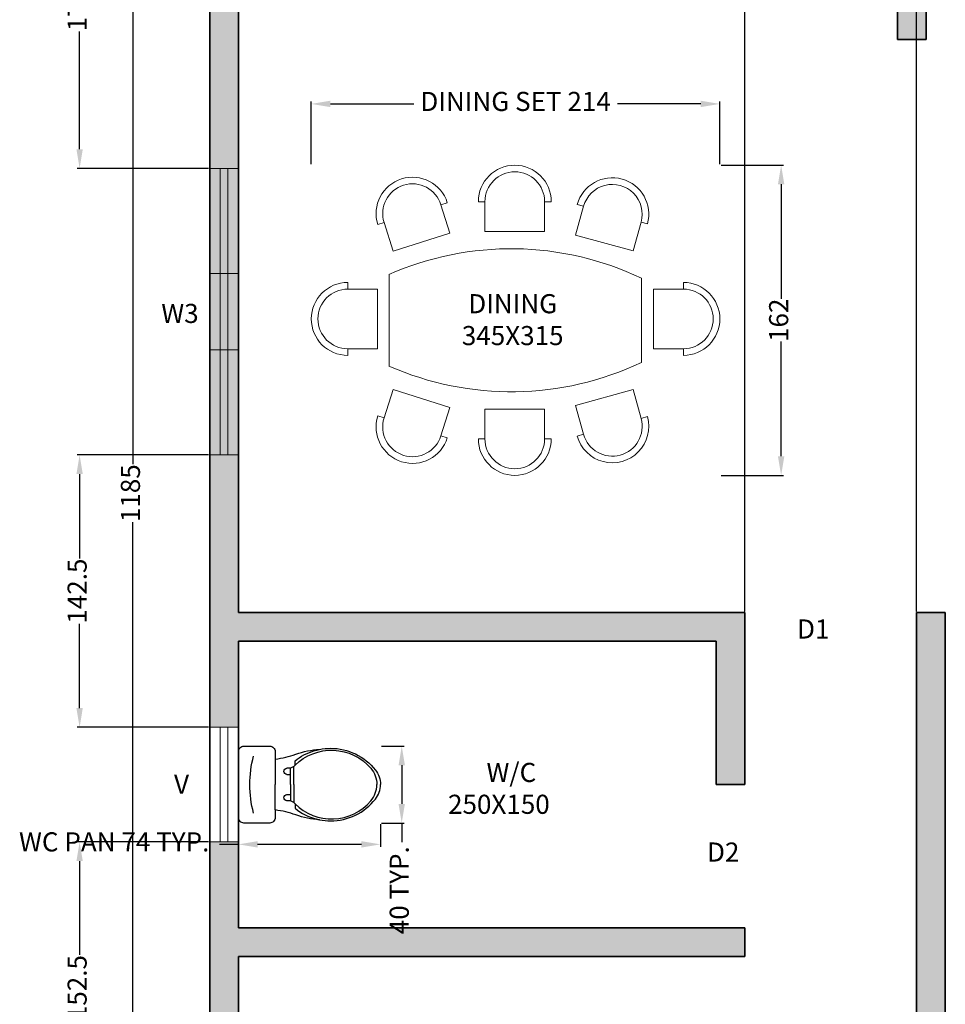
# Model space of a CAD drawing. Units: centimetres. Extents: x 2401 to 3632, y 2122 to 3526.
# Tile 5 of 10: x 2401 to 2885, y 2591 to 3106. Entities that reach past the tile are written whole.
import ezdxf

# ---------------------------------------------------------------- set-up
doc = ezdxf.new("R2010")
doc.units = ezdxf.units.CM
for name, color, linetype, lineweight in [('A-ANNO-DIMS', 9, 'Continuous', 18), ('A-ANNO-TEXT', 9, 'Continuous', 18), ('A-AREA-IDEN', 9, 'Continuous', 25), ('A-FLOR-FIXT', 9, 'Continuous', 18), ('A-FURN', 9, 'Continuous', 18), ('A-GLAZ', 4, 'Continuous', 18), ('A-WALL', 7, 'Continuous', 35)]:
    doc.layers.add(name, color=color, linetype=linetype, lineweight=lineweight)
doc.layers.add('A-GLAZ-PATT', color=251, linetype='Continuous', lineweight=13, true_color=0x636466)
doc.layers.add('A-WALL-PATT', color=18, linetype='Continuous', lineweight=13, true_color=0x000000)
doc.layers.add('WC-Detail_dwgmodels.com', color=251, linetype='Continuous')
doc.layers.add('WC-Outline_dwgmodels.com', color=250, linetype='Continuous')
doc.styles.get("Standard").update_dxf_attribs({"font": 'arial.ttf'})
doc.dimstyles.new('ISO-25', dxfattribs={"dimtxt": 10, "dimasz": 10, "dimexe": 1.25, "dimexo": 0.625, "dimtad": 0, "dimtxsty": 'Standard', "dimcen": 2.5, "dimadec": 0, "dimazin": 0, "dimtfac": 1, "dimtmove": 0, "dimatfit": 3, "dimfxl": 1, "dimarcsym": 0})

# ---------------------------------------------------------------- blocks, each defined once
blk = doc.blocks.new('8 Person Rec 02')
for p, q in [((297.8, 2221.1), (-316.2, 2221.1)), ((-292, 526.8), (273.7, 526.8))]:
    blk.add_line(p, q)
for points in [[(200.3, 2498), (244.8, 2498, 1), (-244.8, 2498), (-200.3, 2498)], [(-664.7, 2254.2), (-651.4, 2296.6, 1), (-798, 1829.6), (-784.7, 1872.1)], [(646.4, 2254.2), (633.1, 2296.6, -1), (779.7, 1829.6), (766.3, 1872.1)], [(-805.2, 1576.8), (-805.2, 1621.3, 1), (-805.2, 1131.8), (-805.2, 1176.3)], [(786.9, 1576.8), (786.9, 1621.3, -1), (786.9, 1131.8), (786.9, 1176.3)], [(-667.7, 528.7), (-655.9, 485.8, -1), (-786.2, 957.6), (-774.3, 914.7)], [(649.4, 528.7), (637.6, 485.8, 1), (767.8, 957.6), (756, 914.7)], [(200.3, 244.8), (244.8, 244.8, -1), (-244.8, 244.8), (-200.3, 244.8)]]:
    blk.add_lwpolyline(points, format="xyb")
for points in [[(-200.3, 2498, -1), (200.3, 2498), (200.3, 2297.7), (-200.3, 2297.7)], [(-664.7, 2254.2, 1), (-784.7, 1872.1), (-593.6, 1812.1), (-473.6, 2194.2)], [(646.4, 2254.2, -1), (766.3, 1872.1), (575.3, 1812.1), (455.3, 2194.2)], [(-805.2, 1176.3), (-605, 1176.3), (-605, 1576.8), (-805.2, 1576.8, 1)], [(786.9, 1176.3), (586.7, 1176.3), (586.7, 1576.8), (786.9, 1576.8, -1)], [(-667.7, 528.7), (-474.7, 582), (-581.3, 968), (-774.3, 914.7, 1)], [(649.4, 528.7), (456.4, 582), (563, 968), (756, 914.7, -1)], [(-200.3, 244.8, 1), (200.3, 244.8), (200.3, 445), (-200.3, 445)]]:
    blk.add_lwpolyline(points, format="xyb", close=True)
for centre, start, end in [((1542.6, 1400.3), 156.17374, 205.45979), ((-1560.9, 1400.3), 334.54021, 23.82626)]:
    blk.add_arc(centre, 2031.9, start, end)
blk = doc.blocks.new('pan')
at = {"layer": 'WC-Detail_dwgmodels.com'}
for p, q in [((2871.96, 3760.91), (2871.96, 3762.74)), ((2875.24, 3762.74), (2875.24, 3760.91)), ((2885.75, 3762.74), (2885.75, 3760.91)), ((2889.03, 3760.91), (2889.03, 3762.74)), ((2871.05, 3759.24), (2871.96, 3760.91)), ((2875.24, 3760.91), (2871.96, 3760.91)), ((2880.5, 3760.91), (2875.24, 3760.91)), ((2880.5, 3760.91), (2885.75, 3760.91)), ((2885.75, 3760.91), (2889.03, 3760.91)), ((2889.94, 3759.24), (2889.03, 3760.91))]:
    blk.add_line(p, q, dxfattribs=at)
for points in [[(2870.35, 3758.55, 0.434217), (2871.96, 3718.84, 0.182634), (2880.5, 3715.73, 2.693815)], [(2868.08, 3758.55, 0.094048), (2862.86, 3748.73, 0.16845)], [(2870.35, 3758.55), (2868.08, 3758.55, 0.416606)], [(2871.05, 3759.24, 0.008985), (2870.35, 3758.55, 0.182634)], [(2880.5, 3759.24), (2871.05, 3759.24, 0.008985)], [(2880.5, 3759.24), (2889.94, 3759.24, -0.444938)], [(2890.64, 3758.55, -0.434217), (2889.03, 3718.84, -0.182634), (2880.5, 3715.73, -2.693815)], [(2889.94, 3759.24, -0.008985), (2890.64, 3758.55, -0.182634)], [(2890.64, 3758.55), (2892.91, 3758.55, -0.416606)], [(2892.91, 3758.55, -0.105447), (2898.5, 3747.44, -0.16845)], [(2862.86, 3748.73, 0.026594), (2862.08, 3745.66, 0.16845)], [(2898.5, 3747.44, -0.015301), (2898.91, 3745.66, -0.16845)]]:
    blk.add_lwpolyline(points, format="xyb", dxfattribs=at)
for centre, radius, start, end in [((2880.52, 3723.1), 59.08, 90.028, 104.6712), ((2880.47, 3723.1), 59.08, 75.3288, 89.972), ((2873.6, 3762.74), 1.64, 0, 180), ((2887.39, 3762.74), 1.64, 0, 180)]:
    blk.add_arc(centre, radius, start, end, dxfattribs=at)
at = {"layer": 'WC-Outline_dwgmodels.com'}
for points in [[(2897.74, 3768.89, 0.414214), (2900.63, 3771.78), (2900.63, 3785.26, 0.414214), (2897.74, 3788.15), (2880.5, 3788.15), (2863.25, 3788.15, 0.414214), (2860.36, 3785.26), (2860.36, 3771.78, 0.414214), (2863.25, 3768.89), (2867.2, 3768.89, -0.052345), (2864.6, 3758.11, 0.071131), (2862.08, 3745.66, 0.160777)], [(2867.2, 3768.89), (2880.5, 3768.89, 0.414214)], [(2893.79, 3768.89), (2880.5, 3768.89, -0.414214)], [(2898.91, 3745.66, 0.071131), (2896.39, 3758.11, -0.052345), (2893.79, 3768.89), (2897.74, 3768.89, 0.414214)], [(2862.08, 3745.66, 0.048023), (2861.52, 3739.97, 0.16845)], [(2898.91, 3745.66, -0.048023), (2899.47, 3739.97, -0.16845)], [(2861.52, 3739.97, 0.230343), (2872.88, 3716.47, 0.16845), (2880.5, 3713.83, 2.883082)], [(2899.47, 3739.97, -0.230343), (2888.11, 3716.47, -0.16845), (2880.5, 3713.83, -2.883082)]]:
    blk.add_lwpolyline(points, format="xyb", dxfattribs=at)
blk = doc.blocks.new('*D12')
at = {"layer": 'A-ANNO-DIMS', "color": 0, "lineweight": -2, "transparency": 16777216}
for p, q in [((2499.81, 3451.1), (2458.94, 3451.1)), ((2460.19, 3441.1), (2460.19, 2873.73)), ((2460.19, 2276.1), (2460.19, 2843.48)), ((2499.81, 2266.1), (2458.94, 2266.1))]:
    blk.add_line(p, q, dxfattribs=at)
at = {"layer": 'A-ANNO-DIMS', "color": 0, "transparency": 16777216}
for points in [[(2458.52, 3441.1), (2461.85, 3441.1), (2460.19, 3451.1)], [(2458.52, 2276.1), (2461.85, 2276.1), (2460.19, 2266.1)]]:
    blk.add_solid(points, dxfattribs=at)
at = {"layer": 'Defpoints', "color": 0, "transparency": 16777216}
for p in [(2500.44, 3451.1), (2460.19, 2266.1), (2500.44, 2266.1)]:
    blk.add_point(p, dxfattribs=at)
at = {"layer": 'A-ANNO-DIMS', "color": 0, "transparency": 16777216, "insert": (2460.19, 2858.6), "char_height": 10, "attachment_point": 5, "rotation": 90}
blk.add_mtext('1185', dxfattribs=at)
blk = doc.blocks.new('WIN-1500-3P')
for p, q in [((0, 15), (0, 0)), ((55, 15), (55, 0)), ((95, 15), (95, 0)), ((150, 15), (150, 0)), ((0, 9.5), (150, 9.5)), ((0, 5.5), (150, 5.5))]:
    blk.add_line(p, q)
blk = doc.blocks.new('VENT-600')
for p, q in [((15, 60), (0, 60)), ((5.5, 60), (5.5, 0)), ((9.5, 60), (9.5, 0)), ((15, 0), (0, 0))]:
    blk.add_line(p, q)
blk = doc.blocks.new('*D26')
at = {"layer": 'A-ANNO-DIMS', "color": 0, "lineweight": -2, "transparency": 16777216}
for p, q in [((2515.44, 2685.34), (2515.44, 2673.57)), ((2589.76, 2685.34), (2589.76, 2673.57)), ((2515.44, 2674.82), (2505.44, 2674.82)), ((2579.76, 2674.82), (2525.44, 2674.82))]:
    blk.add_line(p, q, dxfattribs=at)
at = {"layer": 'A-ANNO-DIMS', "color": 0, "transparency": 16777216}
for points in [[(2525.44, 2676.48), (2525.44, 2673.15), (2515.44, 2674.82)], [(2579.76, 2676.48), (2579.76, 2673.15), (2589.76, 2674.82)]]:
    blk.add_solid(points, dxfattribs=at)
at = {"layer": 'Defpoints', "color": 0, "transparency": 16777216}
for p in [(2515.44, 2685.97), (2589.76, 2685.97), (2515.44, 2674.82)]:
    blk.add_point(p, dxfattribs=at)
at = {"layer": 'A-ANNO-DIMS', "color": 0, "transparency": 16777216, "insert": (2450.39, 2674.82), "char_height": 10, "attachment_point": 5}
blk.add_mtext('WC PAN 74 TYP.', dxfattribs=at)
blk = doc.blocks.new('*D27')
at = {"layer": 'A-ANNO-DIMS', "color": 0, "lineweight": -2, "transparency": 16777216}
for p, q in [((2590.38, 2726.24), (2602.16, 2726.24)), ((2600.91, 2716.24), (2600.91, 2695.97)), ((2590.38, 2685.97), (2602.16, 2685.97)), ((2600.91, 2685.97), (2600.91, 2675.97))]:
    blk.add_line(p, q, dxfattribs=at)
at = {"layer": 'A-ANNO-DIMS', "color": 0, "transparency": 16777216}
for points in [[(2599.24, 2716.24), (2602.57, 2716.24), (2600.91, 2726.24)], [(2599.24, 2695.97), (2602.57, 2695.97), (2600.91, 2685.97)]]:
    blk.add_solid(points, dxfattribs=at)
at = {"layer": 'Defpoints', "color": 0, "transparency": 16777216}
for p in [(2589.76, 2726.24), (2589.76, 2685.97), (2600.91, 2685.97)]:
    blk.add_point(p, dxfattribs=at)
at = {"layer": 'A-ANNO-DIMS', "color": 0, "transparency": 16777216, "insert": (2600.91, 2650.8), "char_height": 10, "attachment_point": 5, "rotation": 90}
blk.add_mtext('40 TYP.', dxfattribs=at)
blk = doc.blocks.new('*D32')
at = {"layer": 'A-ANNO-DIMS', "color": 0, "lineweight": -2, "transparency": 16777216}
for p, q in [((2553.57, 3030.87), (2553.57, 3063.57)), ((2563.57, 3062.32), (2607.18, 3062.32)), ((2757.42, 3062.32), (2713.81, 3062.32)), ((2767.42, 3030.87), (2767.42, 3063.57))]:
    blk.add_line(p, q, dxfattribs=at)
at = {"layer": 'A-ANNO-DIMS', "color": 0, "transparency": 16777216}
for points in [[(2563.57, 3063.99), (2563.57, 3060.65), (2553.57, 3062.32)], [(2757.42, 3063.99), (2757.42, 3060.65), (2767.42, 3062.32)]]:
    blk.add_solid(points, dxfattribs=at)
at = {"layer": 'Defpoints', "color": 0, "transparency": 16777216}
for p in [(2553.57, 3062.32), (2553.57, 3030.24), (2767.42, 3030.24)]:
    blk.add_point(p, dxfattribs=at)
at = {"layer": 'A-ANNO-DIMS', "color": 0, "transparency": 16777216, "insert": (2660.5, 3062.32), "char_height": 10, "attachment_point": 5}
blk.add_mtext('DINING SET 214', dxfattribs=at)
blk = doc.blocks.new('*D33')
at = {"layer": 'A-ANNO-DIMS', "color": 0, "lineweight": -2, "transparency": 16777216}
for p, q in [((2768.05, 3030.24), (2800.75, 3030.24)), ((2799.5, 3020.24), (2799.5, 2960.24)), ((2799.5, 2877.93), (2799.5, 2937.94)), ((2768.05, 2867.93), (2800.75, 2867.93))]:
    blk.add_line(p, q, dxfattribs=at)
at = {"layer": 'A-ANNO-DIMS', "color": 0, "transparency": 16777216}
for points in [[(2797.83, 3020.24), (2801.17, 3020.24), (2799.5, 3030.24)], [(2797.83, 2877.93), (2801.17, 2877.93), (2799.5, 2867.93)]]:
    blk.add_solid(points, dxfattribs=at)
at = {"layer": 'Defpoints', "color": 0, "transparency": 16777216}
for p in [(2767.42, 3030.24), (2799.5, 3030.24), (2767.42, 2867.93)]:
    blk.add_point(p, dxfattribs=at)
at = {"layer": 'A-ANNO-DIMS', "color": 0, "transparency": 16777216, "insert": (2799.5, 2949.09), "char_height": 10, "attachment_point": 5, "rotation": 90}
blk.add_mtext('162', dxfattribs=at)
blk = doc.blocks.new('*D40')
at = {"layer": 'A-ANNO-DIMS', "color": 0, "lineweight": -2, "transparency": 16777216}
for p, q in [((2499.81, 2676.1), (2431.04, 2676.1)), ((2432.29, 2666.1), (2432.29, 2616.92)), ((2432.29, 2533.6), (2432.29, 2582.79)), ((2499.81, 2523.6), (2431.04, 2523.6))]:
    blk.add_line(p, q, dxfattribs=at)
at = {"layer": 'A-ANNO-DIMS', "color": 0, "transparency": 16777216}
for points in [[(2430.62, 2666.1), (2433.95, 2666.1), (2432.29, 2676.1)], [(2430.62, 2533.6), (2433.95, 2533.6), (2432.29, 2523.6)]]:
    blk.add_solid(points, dxfattribs=at)
at = {"layer": 'Defpoints', "color": 0, "transparency": 16777216}
for p in [(2432.29, 2676.1), (2500.44, 2676.1), (2500.44, 2523.6)]:
    blk.add_point(p, dxfattribs=at)
at = {"layer": 'A-ANNO-DIMS', "color": 0, "transparency": 16777216, "insert": (2432.29, 2599.85), "char_height": 10, "attachment_point": 5, "rotation": 90}
blk.add_mtext('152.5', dxfattribs=at)
blk = doc.blocks.new('*D41')
at = {"layer": 'A-ANNO-DIMS', "color": 0, "lineweight": -2, "transparency": 16777216}
for p, q in [((2499.81, 2878.6), (2431.04, 2878.6)), ((2432.29, 2868.6), (2432.29, 2824.42)), ((2432.29, 2746.1), (2432.29, 2790.29)), ((2499.81, 2736.1), (2431.04, 2736.1))]:
    blk.add_line(p, q, dxfattribs=at)
at = {"layer": 'A-ANNO-DIMS', "color": 0, "transparency": 16777216}
for points in [[(2430.62, 2868.6), (2433.95, 2868.6), (2432.29, 2878.6)], [(2430.62, 2746.1), (2433.95, 2746.1), (2432.29, 2736.1)]]:
    blk.add_solid(points, dxfattribs=at)
at = {"layer": 'Defpoints', "color": 0, "transparency": 16777216}
for p in [(2432.29, 2878.6), (2500.44, 2878.6), (2500.44, 2736.1)]:
    blk.add_point(p, dxfattribs=at)
at = {"layer": 'A-ANNO-DIMS', "color": 0, "transparency": 16777216, "insert": (2432.29, 2807.35), "char_height": 10, "attachment_point": 5, "rotation": 90}
blk.add_mtext('142.5', dxfattribs=at)
blk = doc.blocks.new('*D42')
at = {"layer": 'A-ANNO-DIMS', "color": 0, "lineweight": -2, "transparency": 16777216}
for p, q in [((2499.81, 3206.1), (2431.04, 3206.1)), ((2432.29, 3196.1), (2432.29, 3134.42)), ((2432.29, 3038.6), (2432.29, 3100.29)), ((2499.81, 3028.6), (2431.04, 3028.6))]:
    blk.add_line(p, q, dxfattribs=at)
at = {"layer": 'A-ANNO-DIMS', "color": 0, "transparency": 16777216}
for points in [[(2430.62, 3196.1), (2433.95, 3196.1), (2432.29, 3206.1)], [(2430.62, 3038.6), (2433.95, 3038.6), (2432.29, 3028.6)]]:
    blk.add_solid(points, dxfattribs=at)
at = {"layer": 'Defpoints', "color": 0, "transparency": 16777216}
for p in [(2432.29, 3206.1), (2500.44, 3206.1), (2500.44, 3028.6)]:
    blk.add_point(p, dxfattribs=at)
at = {"layer": 'A-ANNO-DIMS', "color": 0, "transparency": 16777216, "insert": (2432.29, 3117.35), "char_height": 10, "attachment_point": 5, "rotation": 90}
blk.add_mtext('177.5', dxfattribs=at)
blk = doc.blocks.new('*D51')
at = {"layer": 'A-ANNO-DIMS', "color": 0, "lineweight": -2, "transparency": 16777216}
for p, q in [((2780.44, 2796.73), (2780.44, 3520.5)), ((2870.44, 2796.73), (2870.44, 3520.5)), ((2790.44, 3519.25), (2817.67, 3519.25)), ((2860.44, 3519.25), (2833.21, 3519.25))]:
    blk.add_line(p, q, dxfattribs=at)
at = {"layer": 'A-ANNO-DIMS', "color": 0, "transparency": 16777216}
for points in [[(2790.44, 3520.92), (2790.44, 3517.59), (2780.44, 3519.25)], [(2860.44, 3520.92), (2860.44, 3517.59), (2870.44, 3519.25)]]:
    blk.add_solid(points, dxfattribs=at)
at = {"layer": 'Defpoints', "color": 0, "transparency": 16777216}
for p in [(2870.44, 3519.25), (2780.44, 2796.1), (2870.44, 2796.1)]:
    blk.add_point(p, dxfattribs=at)
at = {"layer": 'A-ANNO-DIMS', "color": 0, "transparency": 16777216, "insert": (2825.44, 3519.25), "char_height": 10, "attachment_point": 5}
blk.add_mtext('90', dxfattribs=at)

msp = doc.modelspace()

# ---------------------------------------------------------------- hatches: boundary and pattern name
at = {"layer": 'A-GLAZ-PATT'}
h = msp.add_hatch(color=256, dxfattribs=at)
h.dxf.hatch_style = 1
h.paths.add_polyline_path([(2505.936, 3356.104), (2500.436, 3356.104), (2500.436, 3301.104), (2505.936, 3301.104)])
h.paths.add_polyline_path([(2509.936, 3356.104), (2505.936, 3356.104), (2505.936, 3301.104), (2509.936, 3301.104)])
h.paths.add_polyline_path([(2515.436, 3335.674), (2515.436, 3356.104), (2509.936, 3356.104), (2509.936, 3301.104), (2515.436, 3301.104)])
h.paths.add_polyline_path([(2509.936, 3301.104), (2505.936, 3301.104), (2505.936, 3261.104), (2509.936, 3261.104)])
h.paths.add_polyline_path([(2515.436, 3301.104), (2509.936, 3301.104), (2509.936, 3261.104), (2515.436, 3261.104)])
h.paths.add_polyline_path([(2505.936, 3301.104), (2500.436, 3301.104), (2500.436, 3261.104), (2505.936, 3261.104)])
h.paths.add_polyline_path([(2515.436, 3261.104), (2509.936, 3261.104), (2509.936, 3206.104), (2515.436, 3206.104)])
h.paths.add_polyline_path([(2505.936, 3261.104), (2500.436, 3261.104), (2500.436, 3206.104), (2505.936, 3206.104)])
h.paths.add_polyline_path([(2509.936, 3261.104), (2505.936, 3261.104), (2505.936, 3206.104), (2509.936, 3206.104)])
h.paths.add_polyline_path([(3127.936, 3451.104), (3072.936, 3451.104), (3072.936, 3445.604), (3127.936, 3445.604)])
h.paths.add_polyline_path([(3032.936, 3441.604), (2977.936, 3441.604), (2977.936, 3436.104), (3032.936, 3436.104)])
h.paths.add_polyline_path([(3032.936, 3451.104), (2977.936, 3451.104), (2977.936, 3445.604), (3032.936, 3445.604)])
h.paths.add_polyline_path([(3032.936, 3445.604), (2977.936, 3445.604), (2977.936, 3441.604), (3032.936, 3441.604)])
h.paths.add_polyline_path([(3072.936, 3451.104), (3032.936, 3451.104), (3032.936, 3445.604), (3072.936, 3445.604)])
h.paths.add_polyline_path([(3072.936, 3445.604), (3032.936, 3445.604), (3032.936, 3441.604), (3072.936, 3441.604)])
h.paths.add_polyline_path([(3072.936, 3441.604), (3032.936, 3441.604), (3032.936, 3436.104), (3072.936, 3436.104)])
h.paths.add_polyline_path([(3127.936, 3441.604), (3072.936, 3441.604), (3072.936, 3436.104), (3127.936, 3436.104)])
h.paths.add_polyline_path([(3127.936, 3445.604), (3072.936, 3445.604), (3072.936, 3441.604), (3127.936, 3441.604)])
h.paths.add_polyline_path([(3245.436, 3356.104), (3239.936, 3356.104), (3239.936, 3301.104), (3245.436, 3301.104)])
h.paths.add_polyline_path([(3239.936, 3356.104), (3235.936, 3356.104), (3235.936, 3301.104), (3239.936, 3301.104)])
h.paths.add_polyline_path([(3235.936, 3356.104), (3230.436, 3356.104), (3230.436, 3301.104), (3235.936, 3301.104)])
h.paths.add_polyline_path([(3235.936, 3301.104), (3230.436, 3301.104), (3230.436, 3261.104), (3235.936, 3261.104)])
h.paths.add_polyline_path([(3239.936, 3301.104), (3235.936, 3301.104), (3235.936, 3261.104), (3239.936, 3261.104)])
h.paths.add_polyline_path([(3245.436, 3301.104), (3239.936, 3301.104), (3239.936, 3261.104), (3245.436, 3261.104)])
h.paths.add_polyline_path([(3245.436, 3261.104), (3239.936, 3261.104), (3239.936, 3206.104), (3245.436, 3206.104)])
h.paths.add_polyline_path([(3239.936, 3261.104), (3235.936, 3261.104), (3235.936, 3206.104), (3239.936, 3206.104)])
h.paths.add_polyline_path([(3235.936, 3261.104), (3230.436, 3261.104), (3230.436, 3206.104), (3235.936, 3206.104)])
h.paths.add_polyline_path([(3239.936, 3036.104), (3235.936, 3036.104), (3235.936, 2976.104), (3239.936, 2976.104)])
h.paths.add_polyline_path([(3235.936, 3036.104), (3230.436, 3036.104), (3230.436, 2976.104), (3235.936, 2976.104)])
h.paths.add_polyline_path([(3245.436, 3036.104), (3239.936, 3036.104), (3239.936, 2976.104), (3245.436, 2976.104)])
h.paths.add_polyline_path([(3235.936, 2836.104), (3230.436, 2836.104), (3230.436, 2781.104), (3235.936, 2781.104)])
h.paths.add_polyline_path([(3245.436, 2836.104), (3239.936, 2836.104), (3239.936, 2781.104), (3245.436, 2781.104)])
h.paths.add_polyline_path([(3239.936, 2836.104), (3235.936, 2836.104), (3235.936, 2781.104), (3239.936, 2781.104)])
h.paths.add_polyline_path([(3245.436, 2781.104), (3239.936, 2781.104), (3239.936, 2741.104), (3245.436, 2741.104)])
h.paths.add_polyline_path([(3239.936, 2781.104), (3235.936, 2781.104), (3235.936, 2741.104), (3239.936, 2741.104)])
h.paths.add_polyline_path([(3235.936, 2781.104), (3230.436, 2781.104), (3230.436, 2741.104), (3235.936, 2741.104)])
h.paths.add_polyline_path([(3245.436, 2741.104), (3239.936, 2741.104), (3239.936, 2686.104), (3245.436, 2686.104)])
h.paths.add_polyline_path([(3239.936, 2741.104), (3235.936, 2741.104), (3235.936, 2686.104), (3239.936, 2686.104)])
h.paths.add_polyline_path([(3235.936, 2741.104), (3230.436, 2741.104), (3230.436, 2686.104), (3235.936, 2686.104)])
h.paths.add_polyline_path([(3187.936, 2606.104), (3132.936, 2606.104), (3132.936, 2600.604), (3187.936, 2600.604)])
h.paths.add_polyline_path([(3187.936, 2600.604), (3132.936, 2600.604), (3132.936, 2596.604), (3187.936, 2596.604)])
h.paths.add_polyline_path([(3187.936, 2596.604), (3132.936, 2596.604), (3132.936, 2591.104), (3187.936, 2591.104)])
h.paths.add_polyline_path([(3132.936, 2596.604), (3092.936, 2596.604), (3092.936, 2591.104), (3132.936, 2591.104)])
h.paths.add_polyline_path([(3132.936, 2600.604), (3092.936, 2600.604), (3092.936, 2596.604), (3132.936, 2596.604)])
h.paths.add_polyline_path([(3132.936, 2606.104), (3092.936, 2606.104), (3092.936, 2600.604), (3132.936, 2600.604)])
h.paths.add_polyline_path([(3092.936, 2596.604), (3037.936, 2596.604), (3037.936, 2591.104), (3092.936, 2591.104)])
h.paths.add_polyline_path([(3092.936, 2600.604), (3037.936, 2600.604), (3037.936, 2596.604), (3092.936, 2596.604)])
h.paths.add_polyline_path([(3092.936, 2606.104), (3037.936, 2606.104), (3037.936, 2600.604), (3092.936, 2600.604)])
h.paths.add_polyline_path([(2803.613, 3432.66), (2826.471, 3432.66), (2826.471, 3453.267), (2803.613, 3453.267)], flags=9)
h.paths.add_polyline_path([(2904.038, 3087.418), (2926.896, 3087.418), (2926.896, 3108.025), (2904.038, 3108.025)], flags=9)
h.paths.add_polyline_path([(2801.908, 3105.391), (2824.766, 3105.391), (2824.766, 3125.998), (2801.908, 3125.998)], flags=9)
h.paths.add_polyline_path([(2757.576, 2660.284), (2780.434, 2660.284), (2780.434, 2680.892), (2757.576, 2680.892)], flags=9)
h.paths.add_polyline_path([(3004.446, 3080.825), (3027.304, 3080.825), (3027.304, 3101.432), (3004.446, 3101.432)], flags=9)
h.paths.add_polyline_path([(2805.63, 2777.019), (2828.489, 2777.019), (2828.489, 2797.626), (2805.63, 2797.626)], flags=9)
h.paths.add_polyline_path([(3094.334, 2572.754), (3128.823, 2572.754), (3128.823, 2593.361), (3094.334, 2593.361)], flags=9)
h.paths.add_polyline_path([(2931.792, 2588.154), (2946.88, 2588.154), (2946.88, 2608.761), (2931.792, 2608.761)], flags=9)
h.paths.add_polyline_path([(2582.951, 2415.87), (2664.015, 2415.87), (2664.015, 2453.184), (2582.951, 2453.184)], flags=9)
h.paths.add_polyline_path([(2622.234, 2685.113), (2683.168, 2685.113), (2683.168, 2722.427), (2622.234, 2722.427)], flags=9)
h.paths.add_polyline_path([(3027.646, 2511.408), (3088.58, 2511.408), (3088.58, 2548.722), (3027.646, 2548.722)], flags=9)
h.paths.add_polyline_path([(3020.004, 2720.966), (3092.521, 2720.966), (3092.521, 2758.281), (3020.004, 2758.281)], flags=9)
h.paths.add_polyline_path([(2628.506, 2930.416), (2689.441, 2930.416), (2689.441, 2967.73), (2628.506, 2967.73)], flags=9)
h.paths.add_polyline_path([(3056.573, 2986.666), (3117.507, 2986.666), (3117.507, 3023.981), (3056.573, 3023.981)], flags=9)
h.paths.add_polyline_path([(3083.425, 3281.357), (3164.489, 3281.357), (3164.489, 3318.672), (3083.425, 3318.672)], flags=9)
h.paths.add_polyline_path([(2658.367, 3249.15), (2724.683, 3249.15), (2724.683, 3286.465), (2658.367, 3286.465)], flags=9)
h = msp.add_hatch(color=256, dxfattribs=at)
h.dxf.hatch_style = 1
h.paths.add_polyline_path([(3132.936, 2596.604), (3092.936, 2596.604), (3092.936, 2591.104), (3132.936, 2591.104)])
h.paths.add_polyline_path([(2762.936, 2281.104), (2707.936, 2281.104), (2707.936, 2275.604), (2762.936, 2275.604)])
h.paths.add_polyline_path([(2707.936, 2271.604), (2667.936, 2271.604), (2667.936, 2266.104), (2707.936, 2266.104)])
h.paths.add_polyline_path([(2762.936, 2275.604), (2707.936, 2275.604), (2707.936, 2271.604), (2762.936, 2271.604)])
h.paths.add_polyline_path([(2762.936, 2271.604), (2707.936, 2271.604), (2707.936, 2266.104), (2762.936, 2266.104)])
h.paths.add_polyline_path([(2707.936, 2275.604), (2667.936, 2275.604), (2667.936, 2271.604), (2707.936, 2271.604)])
h.paths.add_polyline_path([(2707.936, 2281.104), (2667.936, 2281.104), (2667.936, 2275.604), (2707.936, 2275.604)])
h.paths.add_polyline_path([(2667.936, 2281.104), (2612.936, 2281.104), (2612.936, 2275.604), (2667.936, 2275.604)])
h.paths.add_polyline_path([(2667.936, 2275.604), (2612.936, 2275.604), (2612.936, 2271.604), (2667.936, 2271.604)])
h.paths.add_polyline_path([(2667.936, 2271.604), (2612.936, 2271.604), (2612.936, 2266.104), (2667.936, 2266.104)])
h.paths.add_polyline_path([(2515.436, 2523.604), (2509.936, 2523.604), (2509.936, 2468.604), (2515.436, 2468.604)])
h.paths.add_polyline_path([(2509.936, 2523.604), (2505.936, 2523.604), (2505.936, 2468.604), (2509.936, 2468.604)])
h.paths.add_polyline_path([(2505.936, 2523.604), (2500.436, 2523.604), (2500.436, 2468.604), (2505.936, 2468.604)])
h.paths.add_polyline_path([(2505.936, 2468.604), (2500.436, 2468.604), (2500.436, 2428.604), (2505.936, 2428.604)])
h.paths.add_polyline_path([(2509.936, 2468.604), (2505.936, 2468.604), (2505.936, 2428.604), (2509.936, 2428.604)])
h.paths.add_polyline_path([(2515.436, 2468.604), (2509.936, 2468.604), (2509.936, 2428.604), (2515.436, 2428.604)])
h.paths.add_polyline_path([(2515.436, 2428.604), (2509.936, 2428.604), (2509.936, 2373.604), (2515.436, 2373.604)])
h.paths.add_polyline_path([(2509.936, 2428.604), (2505.936, 2428.604), (2505.936, 2373.604), (2509.936, 2373.604)])
h.paths.add_polyline_path([(2505.936, 2428.604), (2500.436, 2428.604), (2500.436, 2373.604), (2505.936, 2373.604)])
h.paths.add_polyline_path([(2505.936, 3028.604), (2500.436, 3028.604), (2500.436, 2973.604), (2505.936, 2973.604)])
h.paths.add_polyline_path([(2515.436, 3028.604), (2509.936, 3028.604), (2509.936, 2973.604), (2515.436, 2973.604)])
h.paths.add_polyline_path([(2509.936, 3028.604), (2505.936, 3028.604), (2505.936, 2973.604), (2509.936, 2973.604)])
h.paths.add_polyline_path([(2515.436, 2973.604), (2509.936, 2973.604), (2509.936, 2933.604), (2515.436, 2933.604)])
h.paths.add_polyline_path([(2509.936, 2973.604), (2505.936, 2973.604), (2505.936, 2933.604), (2509.936, 2933.604)])
h.paths.add_polyline_path([(2505.936, 2973.604), (2500.436, 2973.604), (2500.436, 2933.604), (2505.936, 2933.604)])
h.paths.add_polyline_path([(2505.936, 2933.604), (2500.436, 2933.604), (2500.436, 2878.604), (2505.936, 2878.604)])
h.paths.add_polyline_path([(2515.436, 2933.604), (2509.936, 2933.604), (2509.936, 2878.604), (2515.436, 2878.604)])
h.paths.add_polyline_path([(2509.936, 2933.604), (2505.936, 2933.604), (2505.936, 2878.604), (2509.936, 2878.604)])
at = {"layer": 'A-WALL-PATT'}
h = msp.add_hatch(color=256, dxfattribs=at)
h.dxf.hatch_style = 1
h.paths.add_polyline_path([(2765.436, 3451.104), (2500.436, 3451.104), (2500.436, 3356.104), (2515.436, 3356.104), (2515.436, 3436.104), (2765.436, 3436.104)])
h.paths.add_polyline_path([(3245.436, 3451.104), (3127.936, 3451.104), (3127.936, 3436.104), (3185.226, 3436.104), (3185.226, 3436.735), (3230.436, 3436.735), (3230.436, 3356.104), (3245.436, 3356.104)])
h.paths.add_polyline_path([(3245.436, 2686.104), (3230.436, 2686.104), (3230.436, 2606.104), (3187.936, 2606.104), (3187.936, 2591.104), (3245.436, 2591.104)])
h.paths.add_polyline_path([(3037.936, 2606.104), (2995.436, 2606.104), (2995.436, 2591.104), (3037.936, 2591.104)])
h.paths.add_polyline_path([(3245.436, 2976.104), (3230.436, 2976.104), (3230.436, 2931.104), (2980.436, 2931.104), (2980.436, 3096.104), (2965.436, 3096.104), (2965.436, 2916.104), (3230.436, 2916.104), (3230.436, 2836.104), (3245.436, 2836.104)])
h.paths.add_polyline_path([(3230.436, 3096.104), (3055.436, 3096.104), (3055.436, 3081.104), (3230.436, 3081.104)], flags=17)
h.paths.add_polyline_path([(2977.936, 3451.104), (2860.436, 3451.104), (2860.436, 3096.104), (2875.436, 3096.104), (2875.436, 3436.104), (2977.936, 3436.104)])
h.paths.add_polyline_path([(2765.436, 3126.104), (2515.436, 3126.104), (2515.436, 3206.104), (2500.436, 3206.104), (2500.436, 3028.604), (2515.436, 3028.604), (2515.436, 3111.104), (2765.436, 3111.104)])
h.paths.add_polyline_path([(2780.436, 2796.104), (2515.436, 2796.104), (2515.436, 2878.604), (2500.436, 2878.604), (2500.436, 2736.104), (2515.436, 2736.104), (2515.436, 2781.104), (2765.436, 2781.104), (2765.436, 2706.104), (2780.436, 2706.104)])
h.paths.add_polyline_path([(2780.436, 2631.104), (2515.436, 2631.104), (2515.436, 2676.104), (2500.436, 2676.104), (2500.436, 2523.604), (2515.436, 2523.604), (2515.436, 2616.104), (2780.436, 2616.104)])
h.paths.add_polyline_path([(2885.436, 2796.104), (2870.436, 2796.104), (2870.436, 2281.104), (2762.936, 2281.104), (2762.936, 2266.104), (2885.436, 2266.104)])
h.paths.add_polyline_path([(2612.936, 2281.104), (2515.436, 2281.104), (2515.436, 2373.604), (2500.436, 2373.604), (2500.436, 2266.104), (2612.936, 2266.104)])

# ---------------------------------------------------------------- linework, layer by layer
at = {"layer": 'A-WALL'}
for p, q in [((2860.436, 3451.104), (2860.436, 3096.104)), ((2875.436, 3436.104), (2875.436, 3096.104)), ((2515.436, 3111.104), (2515.436, 2796.104)), ((2875.436, 3096.104), (2860.436, 3096.104)), ((2780.436, 2796.104), (2515.436, 2796.104)), ((2780.436, 2796.104), (2780.436, 2706.104)), ((2870.436, 2796.104), (2870.436, 2281.104)), ((2870.436, 2796.104), (2885.436, 2796.104)), ((2765.436, 2781.104), (2515.436, 2781.104)), ((2515.436, 2781.104), (2515.436, 2631.104)), ((2765.436, 2781.104), (2765.436, 2706.104)), ((2780.436, 2706.104), (2765.436, 2706.104)), ((2780.436, 2631.104), (2515.436, 2631.104)), ((2780.436, 2631.104), (2780.436, 2616.104)), ((2780.436, 2616.104), (2515.436, 2616.104)), ((2515.436, 2616.104), (2515.436, 2281.104))]:
    msp.add_line(p, q, dxfattribs=at)
msp.add_lwpolyline([(2765.436, 3451.104), (2500.436, 3451.104), (2500.436, 2266.104), (2885.436, 2266.104), (2885.436, 2796.104)], dxfattribs=at)

# ---------------------------------------------------------------- block references
at = {"layer": 'A-FLOR-FIXT', "xscale": -1, "rotation": 90}
msp.add_blockref('pan', (6303.587, 5586.6), dxfattribs=at)
at = {"layer": 'A-FURN', "xscale": 0.0779716797605513, "yscale": 0.0779716797605513, "zscale": 0.0779716797605513, "rotation": 90}
msp.add_blockref('8 Person Rec 02', (2767.423, 2949.802), dxfattribs=at)
at = {"layer": 'A-GLAZ', "rotation": 90.00000000000028}
msp.add_blockref('WIN-1500-3P', (2515.436, 2878.604), dxfattribs=at)
at = {"layer": 'A-GLAZ'}
msp.add_blockref('VENT-600', (2500.436, 2676.104), dxfattribs=at)

# ---------------------------------------------------------------- texts
at = {"layer": 'A-ANNO-TEXT', "char_height": 10, "attachment_point": 1}
for s, width, insert in [('\\pxqc;W3', 66.28614, (2451.681, 2957.674)), ('\\pxqc;D1', 66.28614, (2783.173, 2792.52)), ('\\pxqc;V', 66.28614, (2452.49, 2711.259)), ('\\pxqc;D2', 51.84914, (2743.251, 2675.786))]:
    msp.add_mtext_dynamic_manual_height_columns(s, width=width, gutter_width=12.5, heights=[0], dxfattribs=dict(at, insert=insert))
at = {"layer": 'A-AREA-IDEN', "char_height": 10, "attachment_point": 1}
for s, insert in [('\\pxqc;DINING\\P345X315', (2625.844, 2962.754)), ('\\pxqc;W/C\\P\\pq*;250X150', (2625.143, 2717.451))]:
    msp.add_mtext_dynamic_manual_height_columns(s, width=66.28614, gutter_width=12.5, heights=[0], dxfattribs=dict(at, insert=insert))

# ---------------------------------------------------------------- dimensions: what is measured, and where the dimension line sits
at = {"layer": 'A-ANNO-DIMS'}
dim = msp.add_linear_dim(base=(2870.436, 3519.254), p1=(2780.436, 2796.104), p2=(2870.436, 2796.104), dimstyle='ISO-25', override={"dimdec": 0, "dimlfac": 1, "dimrnd": 0, "dimzin": 0, "dimdsep": 46, "dimlunit": 2}, dxfattribs=at)
dim.commit()
dim.dimension.update_dxf_attribs({"geometry": '*D51', "text_midpoint": (2825.436, 3519.254)})
for base, p1, p2, override, picture, middle in [((2460.187, 2266.104), (2500.436, 3451.104), (2500.436, 2266.104), {"dimclrd": 0, "dimclre": 0, "dimclrt": 0}, '*D12', (2460.187, 2858.604)), ((2432.286, 3206.104), (2500.436, 3028.604), (2500.436, 3206.104), {"dimdec": 1, "dimlfac": 1, "dimrnd": 0, "dimzin": 0, "dimdsep": 46, "dimlunit": 2}, '*D42', (2432.286, 3117.354)), ((2799.501, 3030.242), (2767.423, 2867.932), (2767.423, 3030.242), {"dimdec": 0, "dimlfac": 1, "dimrnd": 0, "dimzin": 0, "dimdsep": 46, "dimlunit": 2}, '*D33', (2799.501, 2949.087)), ((2432.286, 2878.604), (2500.436, 2736.104), (2500.436, 2878.604), {"dimdec": 1, "dimlfac": 1, "dimrnd": 0, "dimzin": 0, "dimdsep": 46, "dimlunit": 2}, '*D41', (2432.286, 2807.354)), ((2432.286, 2676.104), (2500.436, 2523.604), (2500.436, 2676.104), {"dimdec": 1, "dimlfac": 1, "dimrnd": 0, "dimzin": 0, "dimdsep": 46, "dimlunit": 2}, '*D40', (2432.286, 2599.854))]:
    dim = msp.add_linear_dim(base=base, p1=p1, p2=p2, angle=90, dimstyle='ISO-25', override=override, dxfattribs=at)
    dim.commit()
    dim.dimension.update_dxf_attribs({"geometry": picture, "text_midpoint": middle})
for base, p1, p2, angle, text, picture, middle in [((2553.569, 3062.321), (2767.423, 3030.242), (2553.569, 3030.242), 180, 'DINING SET <>', '*D32', (2660.496, 3062.321)), ((2600.906, 2685.966), (2589.758, 2726.243), (2589.758, 2685.966), 270, '<> TYP.', '*D27', (2600.906, 2650.801)), ((2515.436, 2674.817), (2589.758, 2685.966), (2515.436, 2685.966), 180, 'WC PAN <> TYP.', '*D26', (2450.387, 2674.817))]:
    dim = msp.add_linear_dim(base=base, p1=p1, p2=p2, angle=angle, text=text, dimstyle='ISO-25', override={"dimdec": 0, "dimlfac": 1, "dimrnd": 0, "dimzin": 0, "dimdsep": 46, "dimlunit": 2}, dxfattribs=at)
    dim.commit()
    dim.dimension.update_dxf_attribs({"geometry": picture, "text_midpoint": middle})

doc.saveas('drawing.dxf')
